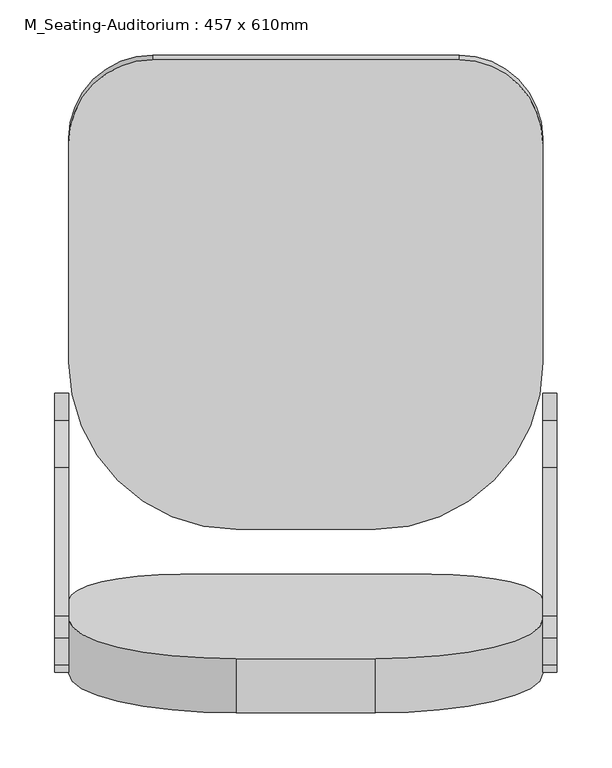
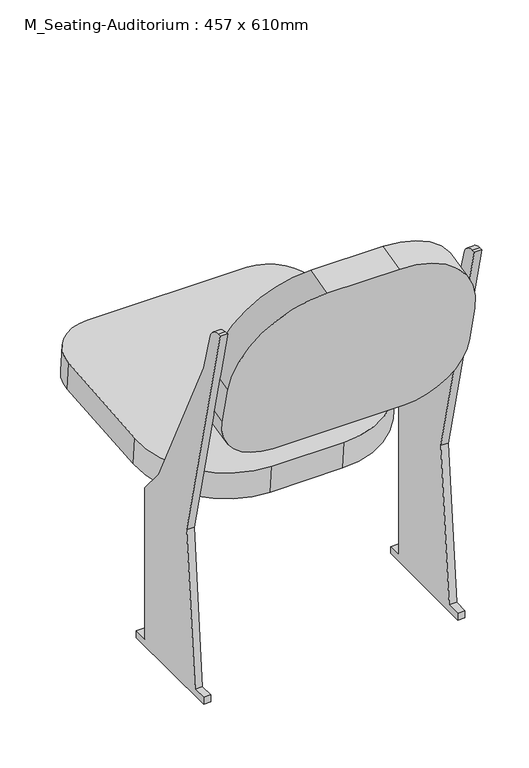
"""IFC4 building model written with IfcOpenShell, lengths in millimetres: furniture geometry, M_Seating-Auditorium : 457 x 610mm."""

from ifc_helpers import new_model, si_unit, point, frame, frame_2d, origin, place, context, project, spatial, polyline, circle_curve, trimmed, segment, composite_curve, outline, extrude, source, transform, mapped, element, save


def m_seating_auditorium_457_x_610mm_eb3a3c23(model_context):
    return source(origin(), model_context, "Body", "SweptSolid", [
        extrude(outline(composite_curve([segment(polyline([(-13.3245902, 12.7), (12.0754098, 12.7), (37.4754098, 292.1), (-64.1245902, 711.2), (-57.883846, 711.2)]), True, "CONTINUOUS"), segment(trimmed(circle_curve(frame_2d((-57.883846, 685.8)), 25.4), [point((-57.883846, 711.2))], [point((-33.4611378, 692.7779166))], False, "CARTESIAN"), True, "CONTINUOUS"), segment(polyline([(-33.4611378, 692.7779166), (-13.3245902, 622.3), (121.8491486, 342.9), (164.4754098, 292.1), (164.4754098, 12.7), (189.8754098, 12.7), (189.8754098, 0.0), (-13.3245902, 0.0), (-13.3245902, 12.7)]), True, "CONTINUOUS")], self_intersect=False)), frame((376.6278689, 0.0, 0.0), z_axis=(1.0, 0.0, 0.0), x_axis=(0.0, 1.0, 0.0)), (0.0, 0.0, 1.0), 12.7),
        extrude(outline(composite_curve([segment(polyline([(-13.3245902, 0.0), (-13.3245902, 12.7), (12.0754098, 12.7), (37.4754098, 292.1), (-64.1245902, 711.2), (-57.883846, 711.2)]), True, "CONTINUOUS"), segment(trimmed(circle_curve(frame_2d((-57.883846, 685.8)), 25.4), [point((-57.883846, 711.2))], [point((-33.4611378, 692.7779166))], False, "CARTESIAN"), True, "CONTINUOUS"), segment(polyline([(-33.4611378, 692.7779166), (-13.3245902, 622.3), (121.8491486, 342.9), (164.4754098, 292.1), (164.4754098, 12.7), (189.8754098, 12.7), (189.8754098, 0.0), (-13.3245902, 0.0)]), True, "CONTINUOUS")], self_intersect=False)), frame((-67.8721311, 0.0, 0.0), z_axis=(1.0, 0.0, 0.0), x_axis=(0.0, 1.0, 0.0)), (0.0, 0.0, 1.0), 12.7),
        extrude(outline(composite_curve([segment(trimmed(circle_curve(frame_2d((0.0, -76.2)), 76.2), [point((0.0, 0.0))], [point((76.2, -76.2))], False, "CARTESIAN"), True, "CONTINUOUS"), segment(polyline([(76.2, -76.2), (76.2, -276.4123505)]), True, "CONTINUOUS"), segment(trimmed(circle_curve(frame_2d((-76.2, -276.4123505)), 152.4), [point((76.2, -276.4123505))], [point((-76.2, -428.8123506))], False, "CARTESIAN"), True, "CONTINUOUS"), segment(polyline([(-76.2, -428.8123506), (-203.2, -428.8123506)]), True, "CONTINUOUS"), segment(trimmed(circle_curve(frame_2d((-203.2, -276.4123505)), 152.4), [point((-203.2, -428.8123506))], [point((-355.6, -276.4123505))], False, "CARTESIAN"), True, "CONTINUOUS"), segment(polyline([(-355.6, -276.4123505), (-355.6, -76.2)]), True, "CONTINUOUS"), segment(trimmed(circle_curve(frame_2d((-279.4, -76.2)), 76.2), [point((-355.6, -76.2))], [point((-279.4, 0.0))], False, "CARTESIAN"), True, "CONTINUOUS"), segment(polyline([(-279.4, 0.0), (0.0, 0.0)]), True, "CONTINUOUS")], self_intersect=False)), frame((300.4278689, 497.5245173, 321.2380213), z_axis=(0.0, -0.08715574274765496, 0.9961946980917459), x_axis=(1.0, 0.0, 0.0)), (0.0, 0.0, 1.0), 50.8),
        extrude(outline(composite_curve([segment(polyline([(0.0, 0.0), (127.0, 0.0)]), True, "CONTINUOUS"), segment(trimmed(circle_curve(frame_2d((127.0, -152.4)), 152.4), [point((127.0, 0.0))], [point((279.4, -152.4))], False, "CARTESIAN"), True, "CONTINUOUS"), segment(polyline([(279.4, -152.4), (279.4, -224.0588601)]), True, "CONTINUOUS"), segment(trimmed(circle_curve(frame_2d((177.8, -224.0588601)), 101.6), [point((279.4, -224.0588601))], [point((177.8, -325.6588601))], False, "CARTESIAN"), True, "CONTINUOUS"), segment(polyline([(177.8, -325.6588601), (-50.8, -325.6588601)]), True, "CONTINUOUS"), segment(trimmed(circle_curve(frame_2d((-50.8, -224.0588601)), 101.6), [point((-50.8, -325.6588601))], [point((-152.4, -224.0588601))], False, "CARTESIAN"), True, "CONTINUOUS"), segment(polyline([(-152.4, -224.0588601), (-152.4, -152.4)]), True, "CONTINUOUS"), segment(trimmed(circle_curve(frame_2d((0.0, -152.4)), 152.4), [point((-152.4, -152.4))], [point((0.0, 0.0))], False, "CARTESIAN"), True, "CONTINUOUS")], self_intersect=False)), frame((224.2278689, -101.3396919, 755.9484479), z_axis=(0.0, 0.9717404775047361, 0.23605178325712217), x_axis=(-1.0, 0.0, 0.0)), (0.0, 0.0, 1.0), 50.8),
    ])


if __name__ == "__main__":
    model = new_model("IFC4")
    model_context = context("Model", 3, world=origin())
    ifc_project = project(units=[si_unit("LENGTHUNIT", "METRE", prefix="MILLI")], contexts=[model_context])
    site = spatial("IfcSite", under=ifc_project)
    building = spatial("IfcBuilding", under=site)
    placement = place(None, origin())
    m_seating_auditorium_457_x_610mm_shape = m_seating_auditorium_457_x_610mm_eb3a3c23(model_context)
    element("IfcFurniture", 1, ObjectType="M_Seating-Auditorium : 457 x 610mm", at=placement, inside=building, context=model_context, shape_type="MappedRepresentation", body=[
        mapped(m_seating_auditorium_457_x_610mm_shape, transform((0.0, 0.0, 0.0), x_axis=(1.0, 0.0, 0.0), y_axis=(0.0, 1.0, 0.0), z_axis=(0.0, 0.0, 1.0))),
    ])
    save(model, "model.ifc")

# Revit data of these elements
# Type "M_Seating-Auditorium : 457 x 610mm"
#   Seat/Back Material = Linen, Beige
#   Frame Material = Steel, Paint Finish, Dark Gray, Matte
#   Default Elevation = 0
# Element 1 (IfcFurniture, "M_Seating-Auditorium : 457 x 610mm")
#   Materials on its faces: "Steel, Paint Finish, Dark Gray, Matte", "Linen, Beige"
# Materials
#   "Linen, Beige": class "Textile", colour RGB 249 239 230, transparency 0, Description = "Linen, beige", Cost = 0
#   "Steel, Paint Finish, Dark Gray, Matte": class "Metal", colour RGB 0 0 0, transparency 0, Description = "Steel, paint finish, dark gray, matte", Cost = 0
